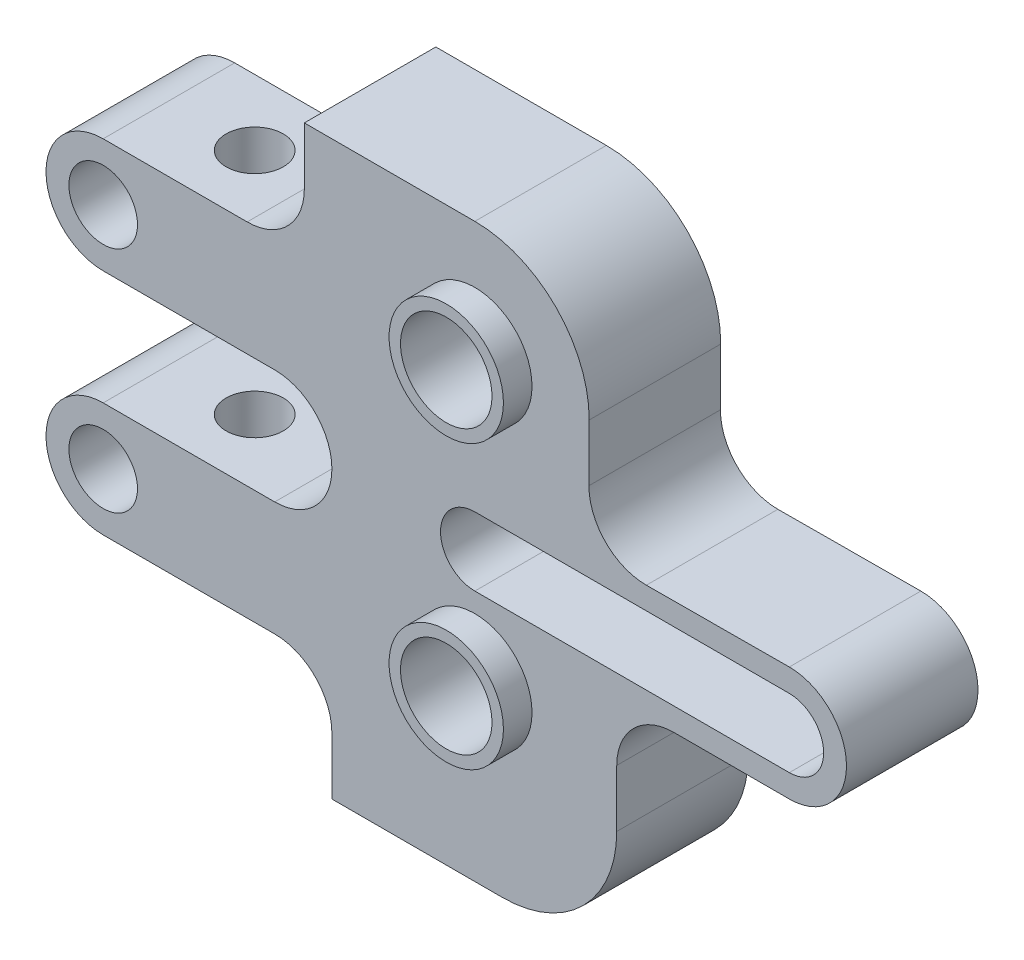
ISO-10303-21;
HEADER;
FILE_DESCRIPTION(('STEP AP214'),'2;1');
FILE_NAME('part.step','',(''),(''),'','','');
FILE_SCHEMA(('AUTOMOTIVE_DESIGN { 1 0 10303 214 1 1 1 1 }'));
ENDSEC;
DATA;
#1=APPLICATION_CONTEXT('core data for automotive mechanical design processes');
#2=APPLICATION_PROTOCOL_DEFINITION('international standard','automotive_design',2000,#1);
#3=PRODUCT_CONTEXT('',#1,'mechanical');
#4=PRODUCT('Part','Part','',(#3));
#5=PRODUCT_RELATED_PRODUCT_CATEGORY('part','',(#4));
#6=PRODUCT_DEFINITION_FORMATION('','',#4);
#7=PRODUCT_DEFINITION_CONTEXT('part definition',#1,'design');
#8=PRODUCT_DEFINITION('design','',#6,#7);
#9=PRODUCT_DEFINITION_SHAPE('','',#8);
#10=(LENGTH_UNIT() NAMED_UNIT(*) SI_UNIT(.MILLI.,.METRE.));
#11=(NAMED_UNIT(*) PLANE_ANGLE_UNIT() SI_UNIT($,.RADIAN.));
#12=(NAMED_UNIT(*) SI_UNIT($,.STERADIAN.) SOLID_ANGLE_UNIT());
#13=UNCERTAINTY_MEASURE_WITH_UNIT(LENGTH_MEASURE(1.E-05),#10,'distance_accuracy_value','');
#14=(GEOMETRIC_REPRESENTATION_CONTEXT(3) GLOBAL_UNCERTAINTY_ASSIGNED_CONTEXT((#13)) GLOBAL_UNIT_ASSIGNED_CONTEXT((#10,
#11,#12)) REPRESENTATION_CONTEXT('',''));
#15=CARTESIAN_POINT('',(0.,0.,0.));
#16=DIRECTION('',(0.,0.,1.));
#17=DIRECTION('',(1.,0.,0.));
#18=AXIS2_PLACEMENT_3D('',#15,#16,#17);
#19=CARTESIAN_POINT('',(120.,-20.,23.));
#20=DIRECTION('',(0.,0.,1.));
#21=DIRECTION('',(1.,0.,0.));
#22=AXIS2_PLACEMENT_3D('',#19,#20,#21);
#23=PLANE('',#22);
#24=CARTESIAN_POINT('',(65.,-39.4111854025044,23.));
#25=DIRECTION('',(0.,0.,1.));
#26=DIRECTION('',(1.,0.,0.));
#27=AXIS2_PLACEMENT_3D('',#24,#25,#26);
#28=CIRCLE('',#27,9.99999999999999);
#29=CARTESIAN_POINT('',(75.,-39.4111854025044,23.));
#30=VERTEX_POINT('',#29);
#31=EDGE_CURVE('E1002',#30,#30,#28,.T.);
#32=ORIENTED_EDGE('',*,*,#31,.F.);
#33=EDGE_LOOP('',(#32));
#34=FACE_BOUND('',#33,.T.);
#35=CARTESIAN_POINT('',(65.,9.99999999999999,23.));
#36=DIRECTION('',(0.,0.,1.));
#37=DIRECTION('',(1.,0.,0.));
#38=AXIS2_PLACEMENT_3D('',#35,#36,#37);
#39=CIRCLE('',#38,10.);
#40=CARTESIAN_POINT('',(75.,9.99999999999999,23.));
#41=VERTEX_POINT('',#40);
#42=EDGE_CURVE('E997',#41,#41,#39,.T.);
#43=ORIENTED_EDGE('',*,*,#42,.F.);
#44=EDGE_LOOP('',(#43));
#45=FACE_BOUND('',#44,.T.);
#46=CARTESIAN_POINT('',(0.,0.,23.));
#47=DIRECTION('',(0.,0.,1.));
#48=DIRECTION('',(1.,0.,0.));
#49=AXIS2_PLACEMENT_3D('',#46,#47,#48);
#50=CIRCLE('',#49,6.);
#51=CARTESIAN_POINT('',(6.,0.,23.));
#52=VERTEX_POINT('',#51);
#53=EDGE_CURVE('E265',#52,#52,#50,.T.);
#54=ORIENTED_EDGE('',*,*,#53,.F.);
#55=EDGE_LOOP('',(#54));
#56=FACE_BOUND('',#55,.T.);
#57=CARTESIAN_POINT('',(120.,-20.,23.));
#58=DIRECTION('',(0.,0.,1.));
#59=DIRECTION('',(1.,0.,0.));
#60=AXIS2_PLACEMENT_3D('',#57,#58,#59);
#61=CIRCLE('',#60,10.);
#62=CARTESIAN_POINT('',(120.,-30.,23.));
#63=VERTEX_POINT('',#62);
#64=CARTESIAN_POINT('',(120.,-10.,23.));
#65=VERTEX_POINT('',#64);
#66=EDGE_CURVE('E268',#63,#65,#61,.T.);
#67=ORIENTED_EDGE('',*,*,#66,.T.);
#68=DIRECTION('',(-0.999989874736936,-0.00450004706711855,0.));
#69=VECTOR('',#68,1.);
#70=CARTESIAN_POINT('',(120.,-10.,23.));
#71=LINE('',#70,#69);
#72=CARTESIAN_POINT('',(95.,-10.1125023157935,23.));
#73=VERTEX_POINT('',#72);
#74=EDGE_CURVE('E271',#65,#73,#71,.T.);
#75=ORIENTED_EDGE('',*,*,#74,.T.);
#76=CARTESIAN_POINT('',(94.9549995293289,-0.112603568423647,23.));
#77=DIRECTION('',(0.,0.,-1.));
#78=DIRECTION('',(-1.,0.,0.));
#79=AXIS2_PLACEMENT_3D('',#76,#77,#78);
#80=CIRCLE('',#79,10.0000000000004);
#81=CARTESIAN_POINT('',(84.9551007777908,-0.0676040240417228,23.));
#82=VERTEX_POINT('',#81);
#83=EDGE_CURVE('E273',#73,#82,#80,.T.);
#84=ORIENTED_EDGE('',*,*,#83,.T.);
#85=DIRECTION('',(0.00449995443819223,0.999989875153771,0.));
#86=VECTOR('',#85,1.);
#87=CARTESIAN_POINT('',(84.955100777791,-0.0676040240417246,23.));
#88=LINE('',#87,#86);
#89=CARTESIAN_POINT('',(84.9999999999997,9.91000091123602,23.));
#90=VERTEX_POINT('',#89);
#91=EDGE_CURVE('E277',#82,#90,#88,.T.);
#92=ORIENTED_EDGE('',*,*,#91,.T.);
#93=CARTESIAN_POINT('',(65.0002024969246,9.99999999999997,23.));
#94=DIRECTION('',(0.,0.,1.));
#95=DIRECTION('',(1.,0.,0.));
#96=AXIS2_PLACEMENT_3D('',#93,#94,#95);
#97=CIRCLE('',#96,19.9999999999997);
#98=CARTESIAN_POINT('',(65.0002024969243,29.9999999999996,23.));
#99=VERTEX_POINT('',#98);
#100=EDGE_CURVE('E279',#90,#99,#97,.T.);
#101=ORIENTED_EDGE('',*,*,#100,.T.);
#102=DIRECTION('',(-1.,1.71333315998742E-11,0.));
#103=VECTOR('',#102,1.);
#104=CARTESIAN_POINT('',(65.,29.9999999999996,23.));
#105=LINE('',#104,#103);
#106=CARTESIAN_POINT('',(35.1799999999999,30.,23.));
#107=VERTEX_POINT('',#106);
#108=EDGE_CURVE('E278',#99,#107,#105,.T.);
#109=ORIENTED_EDGE('',*,*,#108,.T.);
#110=DIRECTION('',(0.,-1.,0.));
#111=VECTOR('',#110,1.);
#112=CARTESIAN_POINT('',(35.1799999999999,20.0000000000001,23.));
#113=LINE('',#112,#111);
#114=CARTESIAN_POINT('',(35.1799999999999,20.0000000000001,23.));
#115=VERTEX_POINT('',#114);
#116=EDGE_CURVE('E285',#107,#115,#113,.T.);
#117=ORIENTED_EDGE('',*,*,#116,.T.);
#118=CARTESIAN_POINT('',(25.1799999999999,20.,23.));
#119=DIRECTION('',(0.,0.,-1.));
#120=DIRECTION('',(-1.,0.,0.));
#121=AXIS2_PLACEMENT_3D('',#118,#119,#120);
#122=CIRCLE('',#121,10.);
#123=CARTESIAN_POINT('',(25.1799999999999,10.,23.));
#124=VERTEX_POINT('',#123);
#125=EDGE_CURVE('E282',#115,#124,#122,.T.);
#126=ORIENTED_EDGE('',*,*,#125,.T.);
#127=DIRECTION('',(-1.,0.,0.));
#128=VECTOR('',#127,1.);
#129=CARTESIAN_POINT('',(0.,10.,23.));
#130=LINE('',#129,#128);
#131=CARTESIAN_POINT('',(0.,10.,23.));
#132=VERTEX_POINT('',#131);
#133=EDGE_CURVE('E286',#124,#132,#130,.T.);
#134=ORIENTED_EDGE('',*,*,#133,.T.);
#135=CARTESIAN_POINT('',(0.,0.,23.));
#136=DIRECTION('',(0.,0.,1.));
#137=DIRECTION('',(1.,0.,0.));
#138=AXIS2_PLACEMENT_3D('',#135,#136,#137);
#139=CIRCLE('',#138,10.);
#140=CARTESIAN_POINT('',(0.,-10.,23.));
#141=VERTEX_POINT('',#140);
#142=EDGE_CURVE('E288',#132,#141,#139,.T.);
#143=ORIENTED_EDGE('',*,*,#142,.T.);
#144=DIRECTION('',(1.,0.,0.));
#145=VECTOR('',#144,1.);
#146=CARTESIAN_POINT('',(0.,-10.,23.));
#147=LINE('',#146,#145);
#148=CARTESIAN_POINT('',(30.,-10.,23.));
#149=VERTEX_POINT('',#148);
#150=EDGE_CURVE('E289',#141,#149,#147,.T.);
#151=ORIENTED_EDGE('',*,*,#150,.T.);
#152=CARTESIAN_POINT('',(30.,-20.,23.));
#153=DIRECTION('',(0.,0.,-1.));
#154=DIRECTION('',(1.,0.,0.));
#155=AXIS2_PLACEMENT_3D('',#152,#153,#154);
#156=CIRCLE('',#155,10.);
#157=CARTESIAN_POINT('',(30.,-30.,23.));
#158=VERTEX_POINT('',#157);
#159=EDGE_CURVE('E295',#149,#158,#156,.T.);
#160=ORIENTED_EDGE('',*,*,#159,.T.);
#161=DIRECTION('',(-1.,0.,0.));
#162=VECTOR('',#161,1.);
#163=CARTESIAN_POINT('',(0.,-30.,23.));
#164=LINE('',#163,#162);
#165=CARTESIAN_POINT('',(0.,-30.,23.));
#166=VERTEX_POINT('',#165);
#167=EDGE_CURVE('E294',#158,#166,#164,.T.);
#168=ORIENTED_EDGE('',*,*,#167,.T.);
#169=CARTESIAN_POINT('',(0.,-40.,23.));
#170=DIRECTION('',(0.,0.,1.));
#171=DIRECTION('',(1.,0.,0.));
#172=AXIS2_PLACEMENT_3D('',#169,#170,#171);
#173=CIRCLE('',#172,10.);
#174=CARTESIAN_POINT('',(0.,-50.,23.));
#175=VERTEX_POINT('',#174);
#176=EDGE_CURVE('E298',#166,#175,#173,.T.);
#177=ORIENTED_EDGE('',*,*,#176,.T.);
#178=DIRECTION('',(1.,0.,0.));
#179=VECTOR('',#178,1.);
#180=CARTESIAN_POINT('',(0.,-50.,23.));
#181=LINE('',#180,#179);
#182=CARTESIAN_POINT('',(29.9999999999999,-50.,23.));
#183=VERTEX_POINT('',#182);
#184=EDGE_CURVE('E296',#175,#183,#181,.T.);
#185=ORIENTED_EDGE('',*,*,#184,.T.);
#186=CARTESIAN_POINT('',(30.,-60.,23.));
#187=DIRECTION('',(0.,0.,-1.));
#188=DIRECTION('',(1.,0.,0.));
#189=AXIS2_PLACEMENT_3D('',#186,#187,#188);
#190=CIRCLE('',#189,10.);
#191=CARTESIAN_POINT('',(40.,-60.0000000000001,23.));
#192=VERTEX_POINT('',#191);
#193=EDGE_CURVE('E299',#183,#192,#190,.T.);
#194=ORIENTED_EDGE('',*,*,#193,.T.);
#195=DIRECTION('',(0.,-1.,0.));
#196=VECTOR('',#195,1.);
#197=CARTESIAN_POINT('',(40.,-60.0000000000001,23.));
#198=LINE('',#197,#196);
#199=CARTESIAN_POINT('',(40.,-70.,23.));
#200=VERTEX_POINT('',#199);
#201=EDGE_CURVE('E305',#192,#200,#198,.T.);
#202=ORIENTED_EDGE('',*,*,#201,.T.);
#203=DIRECTION('',(1.,0.,0.));
#204=VECTOR('',#203,1.);
#205=CARTESIAN_POINT('',(65.,-70.,23.));
#206=LINE('',#205,#204);
#207=CARTESIAN_POINT('',(69.8200000000001,-70.,23.));
#208=VERTEX_POINT('',#207);
#209=EDGE_CURVE('E302',#200,#208,#206,.T.);
#210=ORIENTED_EDGE('',*,*,#209,.T.);
#211=CARTESIAN_POINT('',(69.8200000000001,-50.,23.));
#212=DIRECTION('',(0.,0.,1.));
#213=DIRECTION('',(-1.,0.,0.));
#214=AXIS2_PLACEMENT_3D('',#211,#212,#213);
#215=CIRCLE('',#214,20.);
#216=CARTESIAN_POINT('',(89.8200000000001,-50.,23.));
#217=VERTEX_POINT('',#216);
#218=EDGE_CURVE('E308',#208,#217,#215,.T.);
#219=ORIENTED_EDGE('',*,*,#218,.T.);
#220=DIRECTION('',(0.,1.,0.));
#221=VECTOR('',#220,1.);
#222=CARTESIAN_POINT('',(89.82,-40.,23.));
#223=LINE('',#222,#221);
#224=CARTESIAN_POINT('',(89.82,-40.,23.));
#225=VERTEX_POINT('',#224);
#226=EDGE_CURVE('E306',#217,#225,#223,.T.);
#227=ORIENTED_EDGE('',*,*,#226,.T.);
#228=CARTESIAN_POINT('',(99.8200000000001,-40.,23.));
#229=DIRECTION('',(0.,0.,-1.));
#230=DIRECTION('',(1.,0.,0.));
#231=AXIS2_PLACEMENT_3D('',#228,#229,#230);
#232=CIRCLE('',#231,10.);
#233=CARTESIAN_POINT('',(99.8200000000001,-30.,23.));
#234=VERTEX_POINT('',#233);
#235=EDGE_CURVE('E309',#225,#234,#232,.T.);
#236=ORIENTED_EDGE('',*,*,#235,.T.);
#237=DIRECTION('',(1.,0.,0.));
#238=VECTOR('',#237,1.);
#239=CARTESIAN_POINT('',(120.,-30.,23.));
#240=LINE('',#239,#238);
#241=EDGE_CURVE('E315',#234,#63,#240,.T.);
#242=ORIENTED_EDGE('',*,*,#241,.T.);
#243=EDGE_LOOP('',(#67,#75,#84,#92,#101,#109,#117,#126,#134,#143,#151,#160,#168,#177,#185,#194,
#202,#210,#219,#227,#236,#242));
#244=FACE_BOUND('',#243,.T.);
#245=CARTESIAN_POINT('',(0.,-40.,23.));
#246=DIRECTION('',(0.,0.,1.));
#247=DIRECTION('',(1.,0.,0.));
#248=AXIS2_PLACEMENT_3D('',#245,#246,#247);
#249=CIRCLE('',#248,6.);
#250=CARTESIAN_POINT('',(6.,-40.,23.));
#251=VERTEX_POINT('',#250);
#252=EDGE_CURVE('E258',#251,#251,#249,.T.);
#253=ORIENTED_EDGE('',*,*,#252,.F.);
#254=EDGE_LOOP('',(#253));
#255=FACE_BOUND('',#254,.T.);
#256=DIRECTION('',(-1.,0.,0.));
#257=VECTOR('',#256,1.);
#258=CARTESIAN_POINT('',(120.,-14.,23.));
#259=LINE('',#258,#257);
#260=CARTESIAN_POINT('',(120.,-14.,23.));
#261=VERTEX_POINT('',#260);
#262=CARTESIAN_POINT('',(65.,-14.,23.));
#263=VERTEX_POINT('',#262);
#264=EDGE_CURVE('E228',#261,#263,#259,.T.);
#265=ORIENTED_EDGE('',*,*,#264,.F.);
#266=CARTESIAN_POINT('',(120.,-20.,23.));
#267=DIRECTION('',(0.,0.,1.));
#268=DIRECTION('',(1.,0.,0.));
#269=AXIS2_PLACEMENT_3D('',#266,#267,#268);
#270=CIRCLE('',#269,6.00000000000001);
#271=CARTESIAN_POINT('',(120.,-26.,23.));
#272=VERTEX_POINT('',#271);
#273=EDGE_CURVE('E217',#272,#261,#270,.T.);
#274=ORIENTED_EDGE('',*,*,#273,.F.);
#275=DIRECTION('',(1.,0.,0.));
#276=VECTOR('',#275,1.);
#277=CARTESIAN_POINT('',(120.,-26.,23.));
#278=LINE('',#277,#276);
#279=CARTESIAN_POINT('',(65.,-26.,23.));
#280=VERTEX_POINT('',#279);
#281=EDGE_CURVE('E238',#280,#272,#278,.T.);
#282=ORIENTED_EDGE('',*,*,#281,.F.);
#283=CARTESIAN_POINT('',(65.,-20.,23.));
#284=DIRECTION('',(0.,0.,1.));
#285=DIRECTION('',(1.,0.,0.));
#286=AXIS2_PLACEMENT_3D('',#283,#284,#285);
#287=CIRCLE('',#286,6.);
#288=EDGE_CURVE('E236',#263,#280,#287,.T.);
#289=ORIENTED_EDGE('',*,*,#288,.F.);
#290=EDGE_LOOP('',(#265,#274,#282,#289));
#291=FACE_BOUND('',#290,.T.);
#292=ADVANCED_FACE('F44',(#34,#45,#56,#244,#255,#291),#23,.T.);
#293=CARTESIAN_POINT('',(120.,-20.,0.));
#294=DIRECTION('',(0.,0.,1.));
#295=DIRECTION('',(1.,0.,0.));
#296=AXIS2_PLACEMENT_3D('',#293,#294,#295);
#297=PLANE('',#296);
#298=CARTESIAN_POINT('',(65.,9.99999999999999,0.));
#299=DIRECTION('',(0.,0.,1.));
#300=DIRECTION('',(1.,0.,0.));
#301=AXIS2_PLACEMENT_3D('',#298,#299,#300);
#302=CIRCLE('',#301,8.);
#303=CARTESIAN_POINT('',(73.,9.99999999999999,0.));
#304=VERTEX_POINT('',#303);
#305=EDGE_CURVE('E1024',#304,#304,#302,.T.);
#306=ORIENTED_EDGE('',*,*,#305,.T.);
#307=EDGE_LOOP('',(#306));
#308=FACE_BOUND('',#307,.T.);
#309=CARTESIAN_POINT('',(65.,-39.4111854025044,0.));
#310=DIRECTION('',(0.,0.,1.));
#311=DIRECTION('',(1.,0.,0.));
#312=AXIS2_PLACEMENT_3D('',#309,#310,#311);
#313=CIRCLE('',#312,8.);
#314=CARTESIAN_POINT('',(73.,-39.4111854025044,0.));
#315=VERTEX_POINT('',#314);
#316=EDGE_CURVE('E1028',#315,#315,#313,.T.);
#317=ORIENTED_EDGE('',*,*,#316,.T.);
#318=EDGE_LOOP('',(#317));
#319=FACE_BOUND('',#318,.T.);
#320=CARTESIAN_POINT('',(0.,-40.,0.));
#321=DIRECTION('',(0.,0.,1.));
#322=DIRECTION('',(1.,0.,0.));
#323=AXIS2_PLACEMENT_3D('',#320,#321,#322);
#324=CIRCLE('',#323,6.);
#325=CARTESIAN_POINT('',(6.,-40.,0.));
#326=VERTEX_POINT('',#325);
#327=EDGE_CURVE('E232',#326,#326,#324,.T.);
#328=ORIENTED_EDGE('',*,*,#327,.T.);
#329=EDGE_LOOP('',(#328));
#330=FACE_BOUND('',#329,.T.);
#331=CARTESIAN_POINT('',(0.,0.,0.));
#332=DIRECTION('',(0.,0.,1.));
#333=DIRECTION('',(1.,0.,0.));
#334=AXIS2_PLACEMENT_3D('',#331,#332,#333);
#335=CIRCLE('',#334,6.);
#336=CARTESIAN_POINT('',(6.,0.,0.));
#337=VERTEX_POINT('',#336);
#338=EDGE_CURVE('E259',#337,#337,#335,.T.);
#339=ORIENTED_EDGE('',*,*,#338,.T.);
#340=EDGE_LOOP('',(#339));
#341=FACE_BOUND('',#340,.T.);
#342=CARTESIAN_POINT('',(120.,-20.,0.));
#343=DIRECTION('',(0.,0.,1.));
#344=DIRECTION('',(1.,0.,0.));
#345=AXIS2_PLACEMENT_3D('',#342,#343,#344);
#346=CIRCLE('',#345,10.);
#347=CARTESIAN_POINT('',(120.,-30.,0.));
#348=VERTEX_POINT('',#347);
#349=CARTESIAN_POINT('',(120.,-10.,0.));
#350=VERTEX_POINT('',#349);
#351=EDGE_CURVE('E264',#348,#350,#346,.T.);
#352=ORIENTED_EDGE('',*,*,#351,.F.);
#353=DIRECTION('',(1.,0.,0.));
#354=VECTOR('',#353,1.);
#355=CARTESIAN_POINT('',(120.,-30.,0.));
#356=LINE('',#355,#354);
#357=CARTESIAN_POINT('',(99.8200000000001,-30.,0.));
#358=VERTEX_POINT('',#357);
#359=EDGE_CURVE('E275',#358,#348,#356,.T.);
#360=ORIENTED_EDGE('',*,*,#359,.F.);
#361=CARTESIAN_POINT('',(99.8200000000001,-40.,0.));
#362=DIRECTION('',(0.,0.,-1.));
#363=DIRECTION('',(1.,0.,0.));
#364=AXIS2_PLACEMENT_3D('',#361,#362,#363);
#365=CIRCLE('',#364,10.);
#366=CARTESIAN_POINT('',(89.82,-40.,0.));
#367=VERTEX_POINT('',#366);
#368=EDGE_CURVE('E360',#367,#358,#365,.T.);
#369=ORIENTED_EDGE('',*,*,#368,.F.);
#370=DIRECTION('',(0.,1.,0.));
#371=VECTOR('',#370,1.);
#372=CARTESIAN_POINT('',(89.82,-40.,0.));
#373=LINE('',#372,#371);
#374=CARTESIAN_POINT('',(89.8200000000001,-50.,0.));
#375=VERTEX_POINT('',#374);
#376=EDGE_CURVE('E354',#375,#367,#373,.T.);
#377=ORIENTED_EDGE('',*,*,#376,.F.);
#378=CARTESIAN_POINT('',(69.8200000000001,-50.,0.));
#379=DIRECTION('',(0.,0.,1.));
#380=DIRECTION('',(-1.,0.,0.));
#381=AXIS2_PLACEMENT_3D('',#378,#379,#380);
#382=CIRCLE('',#381,20.);
#383=CARTESIAN_POINT('',(69.8200000000001,-70.,0.));
#384=VERTEX_POINT('',#383);
#385=EDGE_CURVE('E351',#384,#375,#382,.T.);
#386=ORIENTED_EDGE('',*,*,#385,.F.);
#387=DIRECTION('',(1.,0.,0.));
#388=VECTOR('',#387,1.);
#389=CARTESIAN_POINT('',(65.,-70.,0.));
#390=LINE('',#389,#388);
#391=CARTESIAN_POINT('',(40.,-70.,0.));
#392=VERTEX_POINT('',#391);
#393=EDGE_CURVE('E353',#392,#384,#390,.T.);
#394=ORIENTED_EDGE('',*,*,#393,.F.);
#395=DIRECTION('',(0.,-1.,0.));
#396=VECTOR('',#395,1.);
#397=CARTESIAN_POINT('',(40.,-60.0000000000001,0.));
#398=LINE('',#397,#396);
#399=CARTESIAN_POINT('',(40.,-60.0000000000001,0.));
#400=VERTEX_POINT('',#399);
#401=EDGE_CURVE('E346',#400,#392,#398,.T.);
#402=ORIENTED_EDGE('',*,*,#401,.F.);
#403=CARTESIAN_POINT('',(30.,-60.,0.));
#404=DIRECTION('',(0.,0.,-1.));
#405=DIRECTION('',(1.,0.,0.));
#406=AXIS2_PLACEMENT_3D('',#403,#404,#405);
#407=CIRCLE('',#406,10.);
#408=CARTESIAN_POINT('',(29.9999999999999,-50.,0.));
#409=VERTEX_POINT('',#408);
#410=EDGE_CURVE('E347',#409,#400,#407,.T.);
#411=ORIENTED_EDGE('',*,*,#410,.F.);
#412=DIRECTION('',(1.,0.,0.));
#413=VECTOR('',#412,1.);
#414=CARTESIAN_POINT('',(0.,-50.,0.));
#415=LINE('',#414,#413);
#416=CARTESIAN_POINT('',(0.,-50.,0.));
#417=VERTEX_POINT('',#416);
#418=EDGE_CURVE('E342',#417,#409,#415,.T.);
#419=ORIENTED_EDGE('',*,*,#418,.F.);
#420=CARTESIAN_POINT('',(0.,-40.,0.));
#421=DIRECTION('',(0.,0.,1.));
#422=DIRECTION('',(1.,0.,0.));
#423=AXIS2_PLACEMENT_3D('',#420,#421,#422);
#424=CIRCLE('',#423,10.);
#425=CARTESIAN_POINT('',(0.,-30.,0.));
#426=VERTEX_POINT('',#425);
#427=EDGE_CURVE('E345',#426,#417,#424,.T.);
#428=ORIENTED_EDGE('',*,*,#427,.F.);
#429=DIRECTION('',(-1.,0.,0.));
#430=VECTOR('',#429,1.);
#431=CARTESIAN_POINT('',(0.,-30.,0.));
#432=LINE('',#431,#430);
#433=CARTESIAN_POINT('',(30.,-30.,0.));
#434=VERTEX_POINT('',#433);
#435=EDGE_CURVE('E339',#434,#426,#432,.T.);
#436=ORIENTED_EDGE('',*,*,#435,.F.);
#437=CARTESIAN_POINT('',(30.,-20.,0.));
#438=DIRECTION('',(0.,0.,-1.));
#439=DIRECTION('',(1.,0.,0.));
#440=AXIS2_PLACEMENT_3D('',#437,#438,#439);
#441=CIRCLE('',#440,10.);
#442=CARTESIAN_POINT('',(30.,-10.,0.));
#443=VERTEX_POINT('',#442);
#444=EDGE_CURVE('E336',#443,#434,#441,.T.);
#445=ORIENTED_EDGE('',*,*,#444,.F.);
#446=DIRECTION('',(1.,0.,0.));
#447=VECTOR('',#446,1.);
#448=CARTESIAN_POINT('',(0.,-10.,0.));
#449=LINE('',#448,#447);
#450=CARTESIAN_POINT('',(0.,-10.,0.));
#451=VERTEX_POINT('',#450);
#452=EDGE_CURVE('E338',#451,#443,#449,.T.);
#453=ORIENTED_EDGE('',*,*,#452,.F.);
#454=CARTESIAN_POINT('',(0.,0.,0.));
#455=DIRECTION('',(0.,0.,1.));
#456=DIRECTION('',(1.,0.,0.));
#457=AXIS2_PLACEMENT_3D('',#454,#455,#456);
#458=CIRCLE('',#457,10.);
#459=CARTESIAN_POINT('',(0.,10.,0.));
#460=VERTEX_POINT('',#459);
#461=EDGE_CURVE('E331',#460,#451,#458,.T.);
#462=ORIENTED_EDGE('',*,*,#461,.F.);
#463=DIRECTION('',(-1.,0.,0.));
#464=VECTOR('',#463,1.);
#465=CARTESIAN_POINT('',(0.,10.,0.));
#466=LINE('',#465,#464);
#467=CARTESIAN_POINT('',(25.1799999999999,10.,0.));
#468=VERTEX_POINT('',#467);
#469=EDGE_CURVE('E335',#468,#460,#466,.T.);
#470=ORIENTED_EDGE('',*,*,#469,.F.);
#471=CARTESIAN_POINT('',(25.1799999999999,20.,0.));
#472=DIRECTION('',(0.,0.,-1.));
#473=DIRECTION('',(-1.,0.,0.));
#474=AXIS2_PLACEMENT_3D('',#471,#472,#473);
#475=CIRCLE('',#474,10.);
#476=CARTESIAN_POINT('',(35.1799999999999,20.0000000000001,0.));
#477=VERTEX_POINT('',#476);
#478=EDGE_CURVE('E329',#477,#468,#475,.T.);
#479=ORIENTED_EDGE('',*,*,#478,.F.);
#480=DIRECTION('',(0.,-1.,0.));
#481=VECTOR('',#480,1.);
#482=CARTESIAN_POINT('',(35.1799999999999,20.0000000000001,0.));
#483=LINE('',#482,#481);
#484=CARTESIAN_POINT('',(35.1799999999999,30.,0.));
#485=VERTEX_POINT('',#484);
#486=EDGE_CURVE('E327',#485,#477,#483,.T.);
#487=ORIENTED_EDGE('',*,*,#486,.F.);
#488=DIRECTION('',(-1.,0.,0.));
#489=VECTOR('',#488,1.);
#490=CARTESIAN_POINT('',(65.,29.9999999999996,0.));
#491=LINE('',#490,#489);
#492=CARTESIAN_POINT('',(65.0002024969243,29.9999999999996,0.));
#493=VERTEX_POINT('',#492);
#494=EDGE_CURVE('E326',#493,#485,#491,.T.);
#495=ORIENTED_EDGE('',*,*,#494,.F.);
#496=CARTESIAN_POINT('',(65.0002024969246,9.99999999999997,0.));
#497=DIRECTION('',(0.,0.,1.));
#498=DIRECTION('',(1.,0.,0.));
#499=AXIS2_PLACEMENT_3D('',#496,#497,#498);
#500=CIRCLE('',#499,19.9999999999997);
#501=CARTESIAN_POINT('',(84.9999999999997,9.91000091123602,0.));
#502=VERTEX_POINT('',#501);
#503=EDGE_CURVE('E323',#502,#493,#500,.T.);
#504=ORIENTED_EDGE('',*,*,#503,.F.);
#505=DIRECTION('',(0.00449995443819223,0.999989875153771,0.));
#506=VECTOR('',#505,1.);
#507=CARTESIAN_POINT('',(84.955100777791,-0.0676040240417246,0.));
#508=LINE('',#507,#506);
#509=CARTESIAN_POINT('',(84.9551007777908,-0.0676040240417228,0.));
#510=VERTEX_POINT('',#509);
#511=EDGE_CURVE('E321',#510,#502,#508,.T.);
#512=ORIENTED_EDGE('',*,*,#511,.F.);
#513=CARTESIAN_POINT('',(94.9549995293289,-0.112603568423647,0.));
#514=DIRECTION('',(0.,0.,-1.));
#515=DIRECTION('',(-1.,0.,0.));
#516=AXIS2_PLACEMENT_3D('',#513,#514,#515);
#517=CIRCLE('',#516,10.0000000000004);
#518=CARTESIAN_POINT('',(95.,-10.1125023157935,0.));
#519=VERTEX_POINT('',#518);
#520=EDGE_CURVE('E317',#519,#510,#517,.T.);
#521=ORIENTED_EDGE('',*,*,#520,.F.);
#522=DIRECTION('',(-0.999989874736936,-0.00450004706711855,0.));
#523=VECTOR('',#522,1.);
#524=CARTESIAN_POINT('',(120.,-10.,0.));
#525=LINE('',#524,#523);
#526=EDGE_CURVE('E320',#350,#519,#525,.T.);
#527=ORIENTED_EDGE('',*,*,#526,.F.);
#528=EDGE_LOOP('',(#352,#360,#369,#377,#386,#394,#402,#411,#419,#428,#436,#445,#453,#462,#470,
#479,#487,#495,#504,#512,#521,#527));
#529=FACE_BOUND('',#528,.T.);
#530=CARTESIAN_POINT('',(120.,-20.,0.));
#531=DIRECTION('',(0.,0.,1.));
#532=DIRECTION('',(1.,0.,0.));
#533=AXIS2_PLACEMENT_3D('',#530,#531,#532);
#534=CIRCLE('',#533,6.00000000000001);
#535=CARTESIAN_POINT('',(120.,-26.,0.));
#536=VERTEX_POINT('',#535);
#537=CARTESIAN_POINT('',(120.,-14.,0.));
#538=VERTEX_POINT('',#537);
#539=EDGE_CURVE('E68',#536,#538,#534,.T.);
#540=ORIENTED_EDGE('',*,*,#539,.T.);
#541=DIRECTION('',(-1.,0.,0.));
#542=VECTOR('',#541,1.);
#543=CARTESIAN_POINT('',(120.,-14.,0.));
#544=LINE('',#543,#542);
#545=CARTESIAN_POINT('',(65.,-14.,0.));
#546=VERTEX_POINT('',#545);
#547=EDGE_CURVE('E233',#538,#546,#544,.T.);
#548=ORIENTED_EDGE('',*,*,#547,.T.);
#549=CARTESIAN_POINT('',(65.,-20.,0.));
#550=DIRECTION('',(0.,0.,1.));
#551=DIRECTION('',(1.,0.,0.));
#552=AXIS2_PLACEMENT_3D('',#549,#550,#551);
#553=CIRCLE('',#552,6.);
#554=CARTESIAN_POINT('',(65.,-26.,0.));
#555=VERTEX_POINT('',#554);
#556=EDGE_CURVE('E248',#546,#555,#553,.T.);
#557=ORIENTED_EDGE('',*,*,#556,.T.);
#558=DIRECTION('',(1.,0.,0.));
#559=VECTOR('',#558,1.);
#560=CARTESIAN_POINT('',(120.,-26.,0.));
#561=LINE('',#560,#559);
#562=EDGE_CURVE('E230',#555,#536,#561,.T.);
#563=ORIENTED_EDGE('',*,*,#562,.T.);
#564=EDGE_LOOP('',(#540,#548,#557,#563));
#565=FACE_BOUND('',#564,.T.);
#566=ADVANCED_FACE('F427',(#308,#319,#330,#341,#529,#565),#297,.F.);
#567=CARTESIAN_POINT('',(120.,-20.,23.));
#568=DIRECTION('',(0.,0.,-1.));
#569=DIRECTION('',(-1.,0.,0.));
#570=AXIS2_PLACEMENT_3D('',#567,#568,#569);
#571=CYLINDRICAL_SURFACE('',#570,10.);
#572=ORIENTED_EDGE('',*,*,#351,.T.);
#573=DIRECTION('',(0.,0.,-1.));
#574=VECTOR('',#573,1.);
#575=CARTESIAN_POINT('',(120.,-10.,23.));
#576=LINE('',#575,#574);
#577=EDGE_CURVE('E11',#65,#350,#576,.T.);
#578=ORIENTED_EDGE('',*,*,#577,.F.);
#579=ORIENTED_EDGE('',*,*,#66,.F.);
#580=DIRECTION('',(0.,0.,-1.));
#581=VECTOR('',#580,1.);
#582=CARTESIAN_POINT('',(120.,-30.,23.));
#583=LINE('',#582,#581);
#584=EDGE_CURVE('E314',#63,#348,#583,.T.);
#585=ORIENTED_EDGE('',*,*,#584,.T.);
#586=EDGE_LOOP('',(#572,#578,#579,#585));
#587=FACE_BOUND('',#586,.T.);
#588=ADVANCED_FACE('F50',(#587),#571,.T.);
#589=CARTESIAN_POINT('',(120.,-10.,23.));
#590=DIRECTION('',(0.00450004706711855,-0.999989874736936,0.));
#591=DIRECTION('',(0.999989874736936,0.00450004706711855,0.));
#592=AXIS2_PLACEMENT_3D('',#589,#590,#591);
#593=PLANE('',#592);
#594=ORIENTED_EDGE('',*,*,#526,.T.);
#595=DIRECTION('',(0.,0.,-1.));
#596=VECTOR('',#595,1.);
#597=CARTESIAN_POINT('',(95.,-10.1125023157935,23.));
#598=LINE('',#597,#596);
#599=EDGE_CURVE('E52',#73,#519,#598,.T.);
#600=ORIENTED_EDGE('',*,*,#599,.F.);
#601=ORIENTED_EDGE('',*,*,#74,.F.);
#602=ORIENTED_EDGE('',*,*,#577,.T.);
#603=EDGE_LOOP('',(#594,#600,#601,#602));
#604=FACE_BOUND('',#603,.T.);
#605=ADVANCED_FACE('F448',(#604),#593,.F.);
#606=CARTESIAN_POINT('',(94.9549995293289,-0.112603568423647,23.));
#607=DIRECTION('',(0.,0.,-1.));
#608=DIRECTION('',(-1.,0.,0.));
#609=AXIS2_PLACEMENT_3D('',#606,#607,#608);
#610=CYLINDRICAL_SURFACE('',#609,10.0000000000004);
#611=ORIENTED_EDGE('',*,*,#520,.T.);
#612=DIRECTION('',(0.,0.,-1.));
#613=VECTOR('',#612,1.);
#614=CARTESIAN_POINT('',(84.9551007777908,-0.0676040240417228,23.));
#615=LINE('',#614,#613);
#616=EDGE_CURVE('E418',#82,#510,#615,.T.);
#617=ORIENTED_EDGE('',*,*,#616,.F.);
#618=ORIENTED_EDGE('',*,*,#83,.F.);
#619=ORIENTED_EDGE('',*,*,#599,.T.);
#620=EDGE_LOOP('',(#611,#617,#618,#619));
#621=FACE_BOUND('',#620,.T.);
#622=ADVANCED_FACE('F421',(#621),#610,.F.);
#623=CARTESIAN_POINT('',(84.955100777791,-0.0676040240417246,23.));
#624=DIRECTION('',(-0.999989875153771,0.00449995443819223,0.));
#625=DIRECTION('',(-0.00449995443819223,-0.999989875153771,0.));
#626=AXIS2_PLACEMENT_3D('',#623,#624,#625);
#627=PLANE('',#626);
#628=ORIENTED_EDGE('',*,*,#511,.T.);
#629=DIRECTION('',(0.,0.,-1.));
#630=VECTOR('',#629,1.);
#631=CARTESIAN_POINT('',(84.9999999999997,9.91000091123602,23.));
#632=LINE('',#631,#630);
#633=EDGE_CURVE('E413',#90,#502,#632,.T.);
#634=ORIENTED_EDGE('',*,*,#633,.F.);
#635=ORIENTED_EDGE('',*,*,#91,.F.);
#636=ORIENTED_EDGE('',*,*,#616,.T.);
#637=EDGE_LOOP('',(#628,#634,#635,#636));
#638=FACE_BOUND('',#637,.T.);
#639=ADVANCED_FACE('F432',(#638),#627,.F.);
#640=CARTESIAN_POINT('',(65.0002024969246,9.99999999999997,23.));
#641=DIRECTION('',(0.,0.,-1.));
#642=DIRECTION('',(-1.,0.,0.));
#643=AXIS2_PLACEMENT_3D('',#640,#641,#642);
#644=CYLINDRICAL_SURFACE('',#643,19.9999999999997);
#645=ORIENTED_EDGE('',*,*,#503,.T.);
#646=DIRECTION('',(0.,0.,-1.));
#647=VECTOR('',#646,1.);
#648=CARTESIAN_POINT('',(65.0002024969243,29.9999999999996,23.));
#649=LINE('',#648,#647);
#650=EDGE_CURVE('E409',#99,#493,#649,.T.);
#651=ORIENTED_EDGE('',*,*,#650,.F.);
#652=ORIENTED_EDGE('',*,*,#100,.F.);
#653=ORIENTED_EDGE('',*,*,#633,.T.);
#654=EDGE_LOOP('',(#645,#651,#652,#653));
#655=FACE_BOUND('',#654,.T.);
#656=ADVANCED_FACE('F437',(#655),#644,.T.);
#657=CARTESIAN_POINT('',(65.,29.9999999999996,23.));
#658=DIRECTION('',(0.,-1.,0.));
#659=DIRECTION('',(1.,0.,0.));
#660=AXIS2_PLACEMENT_3D('',#657,#658,#659);
#661=PLANE('',#660);
#662=ORIENTED_EDGE('',*,*,#494,.T.);
#663=DIRECTION('',(0.,0.,-1.));
#664=VECTOR('',#663,1.);
#665=CARTESIAN_POINT('',(35.1799999999999,30.,23.));
#666=LINE('',#665,#664);
#667=EDGE_CURVE('E410',#107,#485,#666,.T.);
#668=ORIENTED_EDGE('',*,*,#667,.F.);
#669=ORIENTED_EDGE('',*,*,#108,.F.);
#670=ORIENTED_EDGE('',*,*,#650,.T.);
#671=EDGE_LOOP('',(#662,#668,#669,#670));
#672=FACE_BOUND('',#671,.T.);
#673=ADVANCED_FACE('F526',(#672),#661,.F.);
#674=CARTESIAN_POINT('',(35.1799999999999,20.0000000000001,23.));
#675=DIRECTION('',(1.,0.,0.));
#676=DIRECTION('',(0.,0.,-1.));
#677=AXIS2_PLACEMENT_3D('',#674,#675,#676);
#678=PLANE('',#677);
#679=ORIENTED_EDGE('',*,*,#486,.T.);
#680=DIRECTION('',(0.,0.,-1.));
#681=VECTOR('',#680,1.);
#682=CARTESIAN_POINT('',(35.1799999999999,20.0000000000001,23.));
#683=LINE('',#682,#681);
#684=EDGE_CURVE('E404',#115,#477,#683,.T.);
#685=ORIENTED_EDGE('',*,*,#684,.F.);
#686=ORIENTED_EDGE('',*,*,#116,.F.);
#687=ORIENTED_EDGE('',*,*,#667,.T.);
#688=EDGE_LOOP('',(#679,#685,#686,#687));
#689=FACE_BOUND('',#688,.T.);
#690=ADVANCED_FACE('F524',(#689),#678,.F.);
#691=CARTESIAN_POINT('',(25.1799999999999,20.,23.));
#692=DIRECTION('',(0.,0.,-1.));
#693=DIRECTION('',(-1.,0.,0.));
#694=AXIS2_PLACEMENT_3D('',#691,#692,#693);
#695=CYLINDRICAL_SURFACE('',#694,10.);
#696=ORIENTED_EDGE('',*,*,#478,.T.);
#697=DIRECTION('',(0.,0.,-1.));
#698=VECTOR('',#697,1.);
#699=CARTESIAN_POINT('',(25.1799999999999,10.,23.));
#700=LINE('',#699,#698);
#701=EDGE_CURVE('E402',#124,#468,#700,.T.);
#702=ORIENTED_EDGE('',*,*,#701,.F.);
#703=ORIENTED_EDGE('',*,*,#125,.F.);
#704=ORIENTED_EDGE('',*,*,#684,.T.);
#705=EDGE_LOOP('',(#696,#702,#703,#704));
#706=FACE_BOUND('',#705,.T.);
#707=ADVANCED_FACE('F521',(#706),#695,.F.);
#708=CARTESIAN_POINT('',(0.,10.,23.));
#709=DIRECTION('',(0.,-1.,0.));
#710=DIRECTION('',(0.,0.,-1.));
#711=AXIS2_PLACEMENT_3D('',#708,#709,#710);
#712=PLANE('',#711);
#713=CARTESIAN_POINT('',(15.,10.,11.5));
#714=DIRECTION('',(0.,-1.,0.));
#715=DIRECTION('',(0.,0.,-1.));
#716=AXIS2_PLACEMENT_3D('',#713,#714,#715);
#717=CIRCLE('',#716,5.);
#718=CARTESIAN_POINT('',(15.,10.,6.5));
#719=VERTEX_POINT('',#718);
#720=EDGE_CURVE('E1011',#719,#719,#717,.T.);
#721=ORIENTED_EDGE('',*,*,#720,.T.);
#722=EDGE_LOOP('',(#721));
#723=FACE_BOUND('',#722,.T.);
#724=ORIENTED_EDGE('',*,*,#469,.T.);
#725=DIRECTION('',(0.,0.,-1.));
#726=VECTOR('',#725,1.);
#727=CARTESIAN_POINT('',(0.,10.,23.));
#728=LINE('',#727,#726);
#729=EDGE_CURVE('E398',#132,#460,#728,.T.);
#730=ORIENTED_EDGE('',*,*,#729,.F.);
#731=ORIENTED_EDGE('',*,*,#133,.F.);
#732=ORIENTED_EDGE('',*,*,#701,.T.);
#733=EDGE_LOOP('',(#724,#730,#731,#732));
#734=FACE_BOUND('',#733,.T.);
#735=ADVANCED_FACE('F520',(#723,#734),#712,.F.);
#736=CARTESIAN_POINT('',(0.,0.,23.));
#737=DIRECTION('',(0.,0.,-1.));
#738=DIRECTION('',(-1.,0.,0.));
#739=AXIS2_PLACEMENT_3D('',#736,#737,#738);
#740=CYLINDRICAL_SURFACE('',#739,10.);
#741=ORIENTED_EDGE('',*,*,#461,.T.);
#742=DIRECTION('',(0.,0.,-1.));
#743=VECTOR('',#742,1.);
#744=CARTESIAN_POINT('',(0.,-10.,23.));
#745=LINE('',#744,#743);
#746=EDGE_CURVE('E394',#141,#451,#745,.T.);
#747=ORIENTED_EDGE('',*,*,#746,.F.);
#748=ORIENTED_EDGE('',*,*,#142,.F.);
#749=ORIENTED_EDGE('',*,*,#729,.T.);
#750=EDGE_LOOP('',(#741,#747,#748,#749));
#751=FACE_BOUND('',#750,.T.);
#752=ADVANCED_FACE('F515',(#751),#740,.T.);
#753=CARTESIAN_POINT('',(0.,-10.,23.));
#754=DIRECTION('',(0.,1.,0.));
#755=DIRECTION('',(-1.,0.,0.));
#756=AXIS2_PLACEMENT_3D('',#753,#754,#755);
#757=PLANE('',#756);
#758=CARTESIAN_POINT('',(15.,-10.,11.5));
#759=DIRECTION('',(0.,1.,0.));
#760=DIRECTION('',(-1.,0.,0.));
#761=AXIS2_PLACEMENT_3D('',#758,#759,#760);
#762=CIRCLE('',#761,5.);
#763=CARTESIAN_POINT('',(9.99999999999995,-10.,11.5));
#764=VERTEX_POINT('',#763);
#765=EDGE_CURVE('E1016',#764,#764,#762,.T.);
#766=ORIENTED_EDGE('',*,*,#765,.T.);
#767=EDGE_LOOP('',(#766));
#768=FACE_BOUND('',#767,.T.);
#769=ORIENTED_EDGE('',*,*,#452,.T.);
#770=DIRECTION('',(0.,0.,-1.));
#771=VECTOR('',#770,1.);
#772=CARTESIAN_POINT('',(30.,-10.,23.));
#773=LINE('',#772,#771);
#774=EDGE_CURVE('E395',#149,#443,#773,.T.);
#775=ORIENTED_EDGE('',*,*,#774,.F.);
#776=ORIENTED_EDGE('',*,*,#150,.F.);
#777=ORIENTED_EDGE('',*,*,#746,.T.);
#778=EDGE_LOOP('',(#769,#775,#776,#777));
#779=FACE_BOUND('',#778,.T.);
#780=ADVANCED_FACE('F506',(#768,#779),#757,.F.);
#781=CARTESIAN_POINT('',(30.,-20.,23.));
#782=DIRECTION('',(0.,0.,-1.));
#783=DIRECTION('',(-1.,0.,0.));
#784=AXIS2_PLACEMENT_3D('',#781,#782,#783);
#785=CYLINDRICAL_SURFACE('',#784,10.);
#786=ORIENTED_EDGE('',*,*,#444,.T.);
#787=DIRECTION('',(0.,0.,-1.));
#788=VECTOR('',#787,1.);
#789=CARTESIAN_POINT('',(30.,-30.,23.));
#790=LINE('',#789,#788);
#791=EDGE_CURVE('E386',#158,#434,#790,.T.);
#792=ORIENTED_EDGE('',*,*,#791,.F.);
#793=ORIENTED_EDGE('',*,*,#159,.F.);
#794=ORIENTED_EDGE('',*,*,#774,.T.);
#795=EDGE_LOOP('',(#786,#792,#793,#794));
#796=FACE_BOUND('',#795,.T.);
#797=ADVANCED_FACE('F505',(#796),#785,.F.);
#798=CARTESIAN_POINT('',(0.,-30.,23.));
#799=DIRECTION('',(0.,-1.,0.));
#800=DIRECTION('',(1.,0.,0.));
#801=AXIS2_PLACEMENT_3D('',#798,#799,#800);
#802=PLANE('',#801);
#803=CARTESIAN_POINT('',(15.,-30.,11.5));
#804=DIRECTION('',(0.,-1.,0.));
#805=DIRECTION('',(1.,0.,0.));
#806=AXIS2_PLACEMENT_3D('',#803,#804,#805);
#807=CIRCLE('',#806,5.);
#808=CARTESIAN_POINT('',(20.,-30.,11.5));
#809=VERTEX_POINT('',#808);
#810=EDGE_CURVE('E1017',#809,#809,#807,.T.);
#811=ORIENTED_EDGE('',*,*,#810,.T.);
#812=EDGE_LOOP('',(#811));
#813=FACE_BOUND('',#812,.T.);
#814=ORIENTED_EDGE('',*,*,#435,.T.);
#815=DIRECTION('',(0.,0.,-1.));
#816=VECTOR('',#815,1.);
#817=CARTESIAN_POINT('',(0.,-30.,23.));
#818=LINE('',#817,#816);
#819=EDGE_CURVE('E387',#166,#426,#818,.T.);
#820=ORIENTED_EDGE('',*,*,#819,.F.);
#821=ORIENTED_EDGE('',*,*,#167,.F.);
#822=ORIENTED_EDGE('',*,*,#791,.T.);
#823=EDGE_LOOP('',(#814,#820,#821,#822));
#824=FACE_BOUND('',#823,.T.);
#825=ADVANCED_FACE('F500',(#813,#824),#802,.F.);
#826=CARTESIAN_POINT('',(0.,-40.,23.));
#827=DIRECTION('',(0.,0.,-1.));
#828=DIRECTION('',(-1.,0.,0.));
#829=AXIS2_PLACEMENT_3D('',#826,#827,#828);
#830=CYLINDRICAL_SURFACE('',#829,10.);
#831=ORIENTED_EDGE('',*,*,#427,.T.);
#832=DIRECTION('',(0.,0.,-1.));
#833=VECTOR('',#832,1.);
#834=CARTESIAN_POINT('',(0.,-50.,23.));
#835=LINE('',#834,#833);
#836=EDGE_CURVE('E382',#175,#417,#835,.T.);
#837=ORIENTED_EDGE('',*,*,#836,.F.);
#838=ORIENTED_EDGE('',*,*,#176,.F.);
#839=ORIENTED_EDGE('',*,*,#819,.T.);
#840=EDGE_LOOP('',(#831,#837,#838,#839));
#841=FACE_BOUND('',#840,.T.);
#842=ADVANCED_FACE('F491',(#841),#830,.T.);
#843=CARTESIAN_POINT('',(0.,-50.,23.));
#844=DIRECTION('',(0.,1.,0.));
#845=DIRECTION('',(0.,0.,1.));
#846=AXIS2_PLACEMENT_3D('',#843,#844,#845);
#847=PLANE('',#846);
#848=CARTESIAN_POINT('',(15.,-50.,11.5));
#849=DIRECTION('',(0.,-1.,0.));
#850=DIRECTION('',(0.,0.,-1.));
#851=AXIS2_PLACEMENT_3D('',#848,#849,#850);
#852=CIRCLE('',#851,5.);
#853=CARTESIAN_POINT('',(15.,-50.,6.5));
#854=VERTEX_POINT('',#853);
#855=EDGE_CURVE('E1022',#854,#854,#852,.T.);
#856=ORIENTED_EDGE('',*,*,#855,.F.);
#857=EDGE_LOOP('',(#856));
#858=FACE_BOUND('',#857,.T.);
#859=ORIENTED_EDGE('',*,*,#418,.T.);
#860=DIRECTION('',(0.,0.,-1.));
#861=VECTOR('',#860,1.);
#862=CARTESIAN_POINT('',(29.9999999999999,-50.,23.));
#863=LINE('',#862,#861);
#864=EDGE_CURVE('E379',#183,#409,#863,.T.);
#865=ORIENTED_EDGE('',*,*,#864,.F.);
#866=ORIENTED_EDGE('',*,*,#184,.F.);
#867=ORIENTED_EDGE('',*,*,#836,.T.);
#868=EDGE_LOOP('',(#859,#865,#866,#867));
#869=FACE_BOUND('',#868,.T.);
#870=ADVANCED_FACE('F490',(#858,#869),#847,.F.);
#871=CARTESIAN_POINT('',(30.,-60.,23.));
#872=DIRECTION('',(0.,0.,-1.));
#873=DIRECTION('',(-1.,0.,0.));
#874=AXIS2_PLACEMENT_3D('',#871,#872,#873);
#875=CYLINDRICAL_SURFACE('',#874,10.);
#876=ORIENTED_EDGE('',*,*,#410,.T.);
#877=DIRECTION('',(0.,0.,-1.));
#878=VECTOR('',#877,1.);
#879=CARTESIAN_POINT('',(40.,-60.0000000000001,23.));
#880=LINE('',#879,#878);
#881=EDGE_CURVE('E380',#192,#400,#880,.T.);
#882=ORIENTED_EDGE('',*,*,#881,.F.);
#883=ORIENTED_EDGE('',*,*,#193,.F.);
#884=ORIENTED_EDGE('',*,*,#864,.T.);
#885=EDGE_LOOP('',(#876,#882,#883,#884));
#886=FACE_BOUND('',#885,.T.);
#887=ADVANCED_FACE('F485',(#886),#875,.F.);
#888=CARTESIAN_POINT('',(40.,-60.0000000000001,23.));
#889=DIRECTION('',(1.,0.,0.));
#890=DIRECTION('',(0.,0.,-1.));
#891=AXIS2_PLACEMENT_3D('',#888,#889,#890);
#892=PLANE('',#891);
#893=ORIENTED_EDGE('',*,*,#401,.T.);
#894=DIRECTION('',(0.,0.,-1.));
#895=VECTOR('',#894,1.);
#896=CARTESIAN_POINT('',(40.,-70.,23.));
#897=LINE('',#896,#895);
#898=EDGE_CURVE('E372',#200,#392,#897,.T.);
#899=ORIENTED_EDGE('',*,*,#898,.F.);
#900=ORIENTED_EDGE('',*,*,#201,.F.);
#901=ORIENTED_EDGE('',*,*,#881,.T.);
#902=EDGE_LOOP('',(#893,#899,#900,#901));
#903=FACE_BOUND('',#902,.T.);
#904=ADVANCED_FACE('F478',(#903),#892,.F.);
#905=CARTESIAN_POINT('',(65.,-70.,23.));
#906=DIRECTION('',(0.,1.,0.));
#907=DIRECTION('',(-1.,0.,0.));
#908=AXIS2_PLACEMENT_3D('',#905,#906,#907);
#909=PLANE('',#908);
#910=ORIENTED_EDGE('',*,*,#393,.T.);
#911=DIRECTION('',(0.,0.,-1.));
#912=VECTOR('',#911,1.);
#913=CARTESIAN_POINT('',(69.8200000000001,-70.,23.));
#914=LINE('',#913,#912);
#915=EDGE_CURVE('E371',#208,#384,#914,.T.);
#916=ORIENTED_EDGE('',*,*,#915,.F.);
#917=ORIENTED_EDGE('',*,*,#209,.F.);
#918=ORIENTED_EDGE('',*,*,#898,.T.);
#919=EDGE_LOOP('',(#910,#916,#917,#918));
#920=FACE_BOUND('',#919,.T.);
#921=ADVANCED_FACE('F472',(#920),#909,.F.);
#922=CARTESIAN_POINT('',(69.8200000000001,-50.,23.));
#923=DIRECTION('',(0.,0.,-1.));
#924=DIRECTION('',(-1.,0.,0.));
#925=AXIS2_PLACEMENT_3D('',#922,#923,#924);
#926=CYLINDRICAL_SURFACE('',#925,20.);
#927=ORIENTED_EDGE('',*,*,#385,.T.);
#928=DIRECTION('',(0.,0.,-1.));
#929=VECTOR('',#928,1.);
#930=CARTESIAN_POINT('',(89.8200000000001,-50.,23.));
#931=LINE('',#930,#929);
#932=EDGE_CURVE('E366',#217,#375,#931,.T.);
#933=ORIENTED_EDGE('',*,*,#932,.F.);
#934=ORIENTED_EDGE('',*,*,#218,.F.);
#935=ORIENTED_EDGE('',*,*,#915,.T.);
#936=EDGE_LOOP('',(#927,#933,#934,#935));
#937=FACE_BOUND('',#936,.T.);
#938=ADVANCED_FACE('F470',(#937),#926,.T.);
#939=CARTESIAN_POINT('',(89.82,-40.,23.));
#940=DIRECTION('',(-1.,0.,0.));
#941=DIRECTION('',(0.,-1.,0.));
#942=AXIS2_PLACEMENT_3D('',#939,#940,#941);
#943=PLANE('',#942);
#944=ORIENTED_EDGE('',*,*,#376,.T.);
#945=DIRECTION('',(0.,0.,-1.));
#946=VECTOR('',#945,1.);
#947=CARTESIAN_POINT('',(89.82,-40.,23.));
#948=LINE('',#947,#946);
#949=EDGE_CURVE('E364',#225,#367,#948,.T.);
#950=ORIENTED_EDGE('',*,*,#949,.F.);
#951=ORIENTED_EDGE('',*,*,#226,.F.);
#952=ORIENTED_EDGE('',*,*,#932,.T.);
#953=EDGE_LOOP('',(#944,#950,#951,#952));
#954=FACE_BOUND('',#953,.T.);
#955=ADVANCED_FACE('F465',(#954),#943,.F.);
#956=CARTESIAN_POINT('',(99.8200000000001,-40.,23.));
#957=DIRECTION('',(0.,0.,-1.));
#958=DIRECTION('',(-1.,0.,0.));
#959=AXIS2_PLACEMENT_3D('',#956,#957,#958);
#960=CYLINDRICAL_SURFACE('',#959,10.);
#961=ORIENTED_EDGE('',*,*,#368,.T.);
#962=DIRECTION('',(0.,0.,-1.));
#963=VECTOR('',#962,1.);
#964=CARTESIAN_POINT('',(99.8200000000001,-30.,23.));
#965=LINE('',#964,#963);
#966=EDGE_CURVE('E362',#234,#358,#965,.T.);
#967=ORIENTED_EDGE('',*,*,#966,.F.);
#968=ORIENTED_EDGE('',*,*,#235,.F.);
#969=ORIENTED_EDGE('',*,*,#949,.T.);
#970=EDGE_LOOP('',(#961,#967,#968,#969));
#971=FACE_BOUND('',#970,.T.);
#972=ADVANCED_FACE('F456',(#971),#960,.F.);
#973=CARTESIAN_POINT('',(120.,-30.,23.));
#974=DIRECTION('',(0.,1.,0.));
#975=DIRECTION('',(0.,0.,1.));
#976=AXIS2_PLACEMENT_3D('',#973,#974,#975);
#977=PLANE('',#976);
#978=ORIENTED_EDGE('',*,*,#359,.T.);
#979=ORIENTED_EDGE('',*,*,#584,.F.);
#980=ORIENTED_EDGE('',*,*,#241,.F.);
#981=ORIENTED_EDGE('',*,*,#966,.T.);
#982=EDGE_LOOP('',(#978,#979,#980,#981));
#983=FACE_BOUND('',#982,.T.);
#984=ADVANCED_FACE('F453',(#983),#977,.F.);
#985=CARTESIAN_POINT('',(0.,0.,23.));
#986=DIRECTION('',(0.,0.,-1.));
#987=DIRECTION('',(-1.,0.,0.));
#988=AXIS2_PLACEMENT_3D('',#985,#986,#987);
#989=CYLINDRICAL_SURFACE('',#988,6.);
#990=ORIENTED_EDGE('',*,*,#53,.T.);
#991=EDGE_LOOP('',(#990));
#992=FACE_BOUND('',#991,.T.);
#993=ORIENTED_EDGE('',*,*,#338,.F.);
#994=EDGE_LOOP('',(#993));
#995=FACE_BOUND('',#994,.T.);
#996=ADVANCED_FACE('F552',(#992,#995),#989,.F.);
#997=CARTESIAN_POINT('',(0.,-40.,23.));
#998=DIRECTION('',(0.,0.,-1.));
#999=DIRECTION('',(-1.,0.,0.));
#1000=AXIS2_PLACEMENT_3D('',#997,#998,#999);
#1001=CYLINDRICAL_SURFACE('',#1000,6.);
#1002=ORIENTED_EDGE('',*,*,#252,.T.);
#1003=EDGE_LOOP('',(#1002));
#1004=FACE_BOUND('',#1003,.T.);
#1005=ORIENTED_EDGE('',*,*,#327,.F.);
#1006=EDGE_LOOP('',(#1005));
#1007=FACE_BOUND('',#1006,.T.);
#1008=ADVANCED_FACE('F677',(#1004,#1007),#1001,.F.);
#1009=CARTESIAN_POINT('',(120.,-20.,23.));
#1010=DIRECTION('',(0.,0.,-1.));
#1011=DIRECTION('',(-1.,0.,0.));
#1012=AXIS2_PLACEMENT_3D('',#1009,#1010,#1011);
#1013=CYLINDRICAL_SURFACE('',#1012,6.00000000000001);
#1014=ORIENTED_EDGE('',*,*,#539,.F.);
#1015=DIRECTION('',(0.,0.,-1.));
#1016=VECTOR('',#1015,1.);
#1017=CARTESIAN_POINT('',(120.,-26.,23.));
#1018=LINE('',#1017,#1016);
#1019=EDGE_CURVE('E225',#272,#536,#1018,.T.);
#1020=ORIENTED_EDGE('',*,*,#1019,.F.);
#1021=ORIENTED_EDGE('',*,*,#273,.T.);
#1022=DIRECTION('',(0.,0.,-1.));
#1023=VECTOR('',#1022,1.);
#1024=CARTESIAN_POINT('',(120.,-14.,23.));
#1025=LINE('',#1024,#1023);
#1026=EDGE_CURVE('E222',#261,#538,#1025,.T.);
#1027=ORIENTED_EDGE('',*,*,#1026,.T.);
#1028=EDGE_LOOP('',(#1014,#1020,#1021,#1027));
#1029=FACE_BOUND('',#1028,.T.);
#1030=ADVANCED_FACE('F219',(#1029),#1013,.F.);
#1031=CARTESIAN_POINT('',(120.,-14.,23.));
#1032=DIRECTION('',(0.,-1.,0.));
#1033=DIRECTION('',(1.,0.,0.));
#1034=AXIS2_PLACEMENT_3D('',#1031,#1032,#1033);
#1035=PLANE('',#1034);
#1036=ORIENTED_EDGE('',*,*,#547,.F.);
#1037=ORIENTED_EDGE('',*,*,#1026,.F.);
#1038=ORIENTED_EDGE('',*,*,#264,.T.);
#1039=DIRECTION('',(0.,0.,-1.));
#1040=VECTOR('',#1039,1.);
#1041=CARTESIAN_POINT('',(65.,-14.,23.));
#1042=LINE('',#1041,#1040);
#1043=EDGE_CURVE('E234',#263,#546,#1042,.T.);
#1044=ORIENTED_EDGE('',*,*,#1043,.T.);
#1045=EDGE_LOOP('',(#1036,#1037,#1038,#1044));
#1046=FACE_BOUND('',#1045,.T.);
#1047=ADVANCED_FACE('F229',(#1046),#1035,.T.);
#1048=CARTESIAN_POINT('',(65.,-20.,23.));
#1049=DIRECTION('',(0.,0.,-1.));
#1050=DIRECTION('',(-1.,0.,0.));
#1051=AXIS2_PLACEMENT_3D('',#1048,#1049,#1050);
#1052=CYLINDRICAL_SURFACE('',#1051,6.);
#1053=ORIENTED_EDGE('',*,*,#556,.F.);
#1054=ORIENTED_EDGE('',*,*,#1043,.F.);
#1055=ORIENTED_EDGE('',*,*,#288,.T.);
#1056=DIRECTION('',(0.,0.,-1.));
#1057=VECTOR('',#1056,1.);
#1058=CARTESIAN_POINT('',(65.,-26.,23.));
#1059=LINE('',#1058,#1057);
#1060=EDGE_CURVE('E58',#280,#555,#1059,.T.);
#1061=ORIENTED_EDGE('',*,*,#1060,.T.);
#1062=EDGE_LOOP('',(#1053,#1054,#1055,#1061));
#1063=FACE_BOUND('',#1062,.T.);
#1064=ADVANCED_FACE('F711',(#1063),#1052,.F.);
#1065=CARTESIAN_POINT('',(120.,-26.,23.));
#1066=DIRECTION('',(0.,1.,0.));
#1067=DIRECTION('',(-1.,0.,0.));
#1068=AXIS2_PLACEMENT_3D('',#1065,#1066,#1067);
#1069=PLANE('',#1068);
#1070=ORIENTED_EDGE('',*,*,#562,.F.);
#1071=ORIENTED_EDGE('',*,*,#1060,.F.);
#1072=ORIENTED_EDGE('',*,*,#281,.T.);
#1073=ORIENTED_EDGE('',*,*,#1019,.T.);
#1074=EDGE_LOOP('',(#1070,#1071,#1072,#1073));
#1075=FACE_BOUND('',#1074,.T.);
#1076=ADVANCED_FACE('F725',(#1075),#1069,.T.);
#1077=CARTESIAN_POINT('',(65.,9.99999999999999,28.));
#1078=DIRECTION('',(0.,0.,1.));
#1079=DIRECTION('',(1.,0.,0.));
#1080=AXIS2_PLACEMENT_3D('',#1077,#1078,#1079);
#1081=PLANE('',#1080);
#1082=CARTESIAN_POINT('',(65.,9.99999999999999,28.));
#1083=DIRECTION('',(0.,0.,1.));
#1084=DIRECTION('',(1.,0.,0.));
#1085=AXIS2_PLACEMENT_3D('',#1082,#1083,#1084);
#1086=CIRCLE('',#1085,10.);
#1087=CARTESIAN_POINT('',(75.,9.99999999999999,28.));
#1088=VERTEX_POINT('',#1087);
#1089=EDGE_CURVE('E246',#1088,#1088,#1086,.T.);
#1090=ORIENTED_EDGE('',*,*,#1089,.T.);
#1091=EDGE_LOOP('',(#1090));
#1092=FACE_BOUND('',#1091,.T.);
#1093=CARTESIAN_POINT('',(65.,9.99999999999999,28.));
#1094=DIRECTION('',(0.,0.,1.));
#1095=DIRECTION('',(1.,0.,0.));
#1096=AXIS2_PLACEMENT_3D('',#1093,#1094,#1095);
#1097=CIRCLE('',#1096,8.);
#1098=CARTESIAN_POINT('',(73.,9.99999999999999,28.));
#1099=VERTEX_POINT('',#1098);
#1100=EDGE_CURVE('E996',#1099,#1099,#1097,.T.);
#1101=ORIENTED_EDGE('',*,*,#1100,.F.);
#1102=EDGE_LOOP('',(#1101));
#1103=FACE_BOUND('',#1102,.T.);
#1104=ADVANCED_FACE('F731',(#1092,#1103),#1081,.T.);
#1105=CARTESIAN_POINT('',(65.,9.99999999999999,28.));
#1106=DIRECTION('',(0.,0.,-1.));
#1107=DIRECTION('',(-1.,0.,0.));
#1108=AXIS2_PLACEMENT_3D('',#1105,#1106,#1107);
#1109=CYLINDRICAL_SURFACE('',#1108,10.);
#1110=ORIENTED_EDGE('',*,*,#1089,.F.);
#1111=EDGE_LOOP('',(#1110));
#1112=FACE_BOUND('',#1111,.T.);
#1113=ORIENTED_EDGE('',*,*,#42,.T.);
#1114=EDGE_LOOP('',(#1113));
#1115=FACE_BOUND('',#1114,.T.);
#1116=ADVANCED_FACE('F753',(#1112,#1115),#1109,.T.);
#1117=CARTESIAN_POINT('',(65.,9.99999999999999,28.));
#1118=DIRECTION('',(0.,0.,-1.));
#1119=DIRECTION('',(-1.,0.,0.));
#1120=AXIS2_PLACEMENT_3D('',#1117,#1118,#1119);
#1121=CYLINDRICAL_SURFACE('',#1120,8.);
#1122=ORIENTED_EDGE('',*,*,#1100,.T.);
#1123=EDGE_LOOP('',(#1122));
#1124=FACE_BOUND('',#1123,.T.);
#1125=ORIENTED_EDGE('',*,*,#305,.F.);
#1126=EDGE_LOOP('',(#1125));
#1127=FACE_BOUND('',#1126,.T.);
#1128=ADVANCED_FACE('F748',(#1124,#1127),#1121,.F.);
#1129=CARTESIAN_POINT('',(65.,-39.4111854025044,28.));
#1130=DIRECTION('',(0.,0.,1.));
#1131=DIRECTION('',(1.,0.,0.));
#1132=AXIS2_PLACEMENT_3D('',#1129,#1130,#1131);
#1133=PLANE('',#1132);
#1134=CARTESIAN_POINT('',(65.,-39.4111854025044,28.));
#1135=DIRECTION('',(0.,0.,1.));
#1136=DIRECTION('',(1.,0.,0.));
#1137=AXIS2_PLACEMENT_3D('',#1134,#1135,#1136);
#1138=CIRCLE('',#1137,9.99999999999999);
#1139=CARTESIAN_POINT('',(75.,-39.4111854025044,28.));
#1140=VERTEX_POINT('',#1139);
#1141=EDGE_CURVE('E999',#1140,#1140,#1138,.T.);
#1142=ORIENTED_EDGE('',*,*,#1141,.T.);
#1143=EDGE_LOOP('',(#1142));
#1144=FACE_BOUND('',#1143,.T.);
#1145=CARTESIAN_POINT('',(65.,-39.4111854025044,28.));
#1146=DIRECTION('',(0.,0.,1.));
#1147=DIRECTION('',(1.,0.,0.));
#1148=AXIS2_PLACEMENT_3D('',#1145,#1146,#1147);
#1149=CIRCLE('',#1148,8.00000000000001);
#1150=CARTESIAN_POINT('',(73.,-39.4111854025044,28.));
#1151=VERTEX_POINT('',#1150);
#1152=EDGE_CURVE('E1009',#1151,#1151,#1149,.T.);
#1153=ORIENTED_EDGE('',*,*,#1152,.F.);
#1154=EDGE_LOOP('',(#1153));
#1155=FACE_BOUND('',#1154,.T.);
#1156=ADVANCED_FACE('F749',(#1144,#1155),#1133,.T.);
#1157=CARTESIAN_POINT('',(65.,-39.4111854025044,28.));
#1158=DIRECTION('',(0.,0.,-1.));
#1159=DIRECTION('',(-1.,0.,0.));
#1160=AXIS2_PLACEMENT_3D('',#1157,#1158,#1159);
#1161=CYLINDRICAL_SURFACE('',#1160,9.99999999999999);
#1162=ORIENTED_EDGE('',*,*,#1141,.F.);
#1163=EDGE_LOOP('',(#1162));
#1164=FACE_BOUND('',#1163,.T.);
#1165=ORIENTED_EDGE('',*,*,#31,.T.);
#1166=EDGE_LOOP('',(#1165));
#1167=FACE_BOUND('',#1166,.T.);
#1168=ADVANCED_FACE('F762',(#1164,#1167),#1161,.T.);
#1169=CARTESIAN_POINT('',(65.,-39.4111854025044,28.));
#1170=DIRECTION('',(0.,0.,-1.));
#1171=DIRECTION('',(-1.,0.,0.));
#1172=AXIS2_PLACEMENT_3D('',#1169,#1170,#1171);
#1173=CYLINDRICAL_SURFACE('',#1172,8.00000000000001);
#1174=ORIENTED_EDGE('',*,*,#1152,.T.);
#1175=EDGE_LOOP('',(#1174));
#1176=FACE_BOUND('',#1175,.T.);
#1177=ORIENTED_EDGE('',*,*,#316,.F.);
#1178=EDGE_LOOP('',(#1177));
#1179=FACE_BOUND('',#1178,.T.);
#1180=ADVANCED_FACE('F759',(#1176,#1179),#1173,.F.);
#1181=CARTESIAN_POINT('',(15.,30.,11.5));
#1182=DIRECTION('',(0.,-1.,0.));
#1183=DIRECTION('',(0.,0.,-1.));
#1184=AXIS2_PLACEMENT_3D('',#1181,#1182,#1183);
#1185=CYLINDRICAL_SURFACE('',#1184,5.);
#1186=ORIENTED_EDGE('',*,*,#855,.T.);
#1187=EDGE_LOOP('',(#1186));
#1188=FACE_BOUND('',#1187,.T.);
#1189=ORIENTED_EDGE('',*,*,#810,.F.);
#1190=EDGE_LOOP('',(#1189));
#1191=FACE_BOUND('',#1190,.T.);
#1192=ADVANCED_FACE('F763',(#1188,#1191),#1185,.F.);
#1193=ORIENTED_EDGE('',*,*,#765,.F.);
#1194=EDGE_LOOP('',(#1193));
#1195=FACE_BOUND('',#1194,.T.);
#1196=ORIENTED_EDGE('',*,*,#720,.F.);
#1197=EDGE_LOOP('',(#1196));
#1198=FACE_BOUND('',#1197,.T.);
#1199=ADVANCED_FACE('F773',(#1195,#1198),#1185,.F.);
#1200=CLOSED_SHELL('',(#292,#566,#588,#605,#622,#639,#656,#673,#690,#707,#735,#752,#780,#797,
#825,#842,#870,#887,#904,#921,#938,#955,#972,#984,#996,#1008,#1030,#1047,#1064,#1076,#1104,
#1116,#1128,#1156,#1168,#1180,#1192,#1199));
#1201=MANIFOLD_SOLID_BREP('B2',#1200);
#1202=ADVANCED_BREP_SHAPE_REPRESENTATION('',(#18,#1201),#14);
#1203=SHAPE_DEFINITION_REPRESENTATION(#9,#1202);
ENDSEC;
END-ISO-10303-21;
